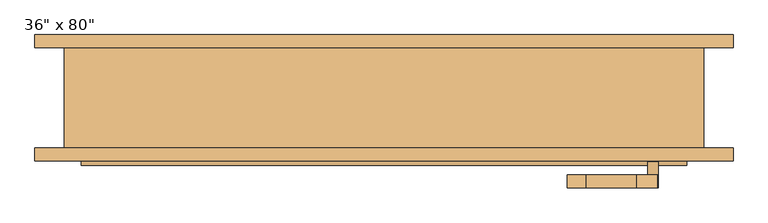
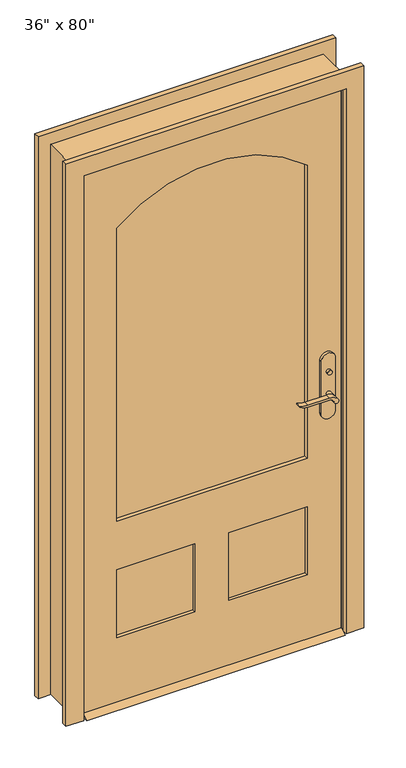
"""IFC4 building model written with IfcOpenShell, lengths in millimetres: door geometry."""

from ifc_helpers import new_model, si_unit, point, frame, frame_2d, origin, place, context, project, spatial, polyline, circle_curve, trimmed, segment, composite_curve, outline, extrude, faceted_brep, source, transform, mapped, element, save


def door_5d363d20(model_context):
    return source(origin(), model_context, "Body", "SolidModel", [
        extrude(outline(polyline([(-38.1, 12.7), (-12.7, 0.0), (-98.425, 0.0), (-73.025, 12.7), (-38.1, 12.7)])), frame((-457.2, 0.0, 0.0), z_axis=(1.0, 0.0, 0.0), x_axis=(0.0, 1.0, 0.0)), (0.0, 0.0, 1.0), 914.4),
        extrude(outline(polyline([(411.4, -18.1), (411.4, -28.1), (401.4, -28.1), (401.4, -18.1), (411.4, -18.1)])), frame((0.0, 0.0, 981.9), z_axis=(0.0, 0.0, 1.0), x_axis=(1.0, 0.0, 0.0)), (0.0, 0.0, 1.0), 30.0),
        extrude(outline(composite_curve([segment(trimmed(circle_curve(frame_2d((996.9, 406.4)), 8.0), [point((996.9, 398.4))], [point((996.9, 414.4))], False, "CARTESIAN"), True, "CONTINUOUS"), segment(trimmed(circle_curve(frame_2d((996.9, 406.4)), 8.0), [point((996.9, 414.4))], [point((996.9, 398.4))], False, "CARTESIAN"), True, "CONTINUOUS")], self_intersect=False)), frame((0.0, -93.025, 0.0), z_axis=(0.0, 1.0, 0.0), x_axis=(0.0, 0.0, 1.0)), (0.0, 0.0, 1.0), 10.0),
        extrude(outline(composite_curve([segment(trimmed(circle_curve(frame_2d((897.1555521, 382.7324871)), 37.2832219), [point((919.0523287, 412.9081363))], [point((934.4, 381.0325667))], False, "CARTESIAN"), True, "CONTINUOUS"), segment(polyline([(934.4, 381.0325667), (934.4, 304.7564091)]), True, "CONTINUOUS"), segment(trimmed(circle_curve(frame_2d((1017.6850638, 304.8227909)), 83.2850902), [point((934.4, 304.7564091))], [point((939.4, 276.4))], True, "CARTESIAN"), True, "CONTINUOUS"), segment(polyline([(939.4, 276.4), (936.6135558, 276.4)]), True, "CONTINUOUS"), segment(trimmed(circle_curve(frame_2d((986.6709207, 308.3396612)), 59.3791355), [point((936.6135558, 276.4))], [point((927.4, 304.7564091))], False, "CARTESIAN"), True, "CONTINUOUS"), segment(polyline([(927.4, 304.7564091), (927.4, 381.0138099)]), True, "CONTINUOUS"), segment(trimmed(circle_curve(frame_2d((909.2738613, 381.0138099)), 18.1261387), [point((927.4, 381.0138099))], [point((914.4, 398.4))], True, "CARTESIAN"), True, "CONTINUOUS"), segment(trimmed(circle_curve(frame_2d((914.4, 406.4)), 8.0), [point((914.4, 398.4))], [point((919.0523287, 412.9081363))], False, "CARTESIAN"), True, "CONTINUOUS")], self_intersect=False)), frame((0.0, 1.9, 0.0), z_axis=(0.0, 1.0, 0.0), x_axis=(0.0, 0.0, 1.0)), (0.0, 0.0, 1.0), 20.0),
        extrude(outline(composite_curve([segment(trimmed(circle_curve(frame_2d((914.4, 406.4)), 8.0), [point((914.3999903, 398.4))], [point((919.0523287, 412.9081363))], False, "CARTESIAN"), True, "CONTINUOUS"), segment(trimmed(circle_curve(frame_2d((897.1555521, 382.7324871)), 37.2832219), [point((919.0523287, 412.9081363))], [point((934.4, 381.0325667))], False, "CARTESIAN"), True, "CONTINUOUS"), segment(polyline([(934.4, 381.0325667), (934.4, 304.7564091)]), True, "CONTINUOUS"), segment(trimmed(circle_curve(frame_2d((1017.6850638, 304.8227909)), 83.2850902), [point((934.4, 304.7564091))], [point((939.4, 276.4))], True, "CARTESIAN"), True, "CONTINUOUS"), segment(polyline([(939.4, 276.4), (936.6135558, 276.4)]), True, "CONTINUOUS"), segment(trimmed(circle_curve(frame_2d((986.6709207, 308.3396612)), 59.3791355), [point((936.6135558, 276.4))], [point((927.4, 304.7564091))], False, "CARTESIAN"), True, "CONTINUOUS"), segment(polyline([(927.4, 304.7564091), (927.4, 381.0138122)]), True, "CONTINUOUS"), segment(trimmed(circle_curve(frame_2d((909.2738682, 381.0138122)), 18.1261318), [point((927.4, 381.0138122))], [point((914.3999903, 398.4))], True, "CARTESIAN"), True, "CONTINUOUS")], self_intersect=False)), frame((0.0, -133.025, 0.0), z_axis=(0.0, 1.0, 0.0), x_axis=(0.0, 0.0, 1.0)), (0.0, 0.0, 1.0), 20.0),
        extrude(outline(composite_curve([segment(trimmed(circle_curve(frame_2d((914.4, 406.4)), 8.0), [point((914.4, 398.4))], [point((914.4, 414.4))], False, "CARTESIAN"), True, "CONTINUOUS"), segment(trimmed(circle_curve(frame_2d((914.4, 406.4)), 8.0), [point((914.4, 414.4))], [point((914.4, 398.4))], False, "CARTESIAN"), True, "CONTINUOUS")], self_intersect=False)), frame((0.0, -28.1, 0.0), z_axis=(0.0, 1.0, 0.0), x_axis=(0.0, 0.0, 1.0)), (0.0, 0.0, 1.0), 30.0),
        extrude(outline(composite_curve([segment(trimmed(circle_curve(frame_2d((914.4, 406.4)), 8.0), [point((914.4, 398.4))], [point((914.4, 414.4))], False, "CARTESIAN"), True, "CONTINUOUS"), segment(trimmed(circle_curve(frame_2d((914.4, 406.4)), 8.0), [point((914.4, 414.4))], [point((914.4, 398.4))], False, "CARTESIAN"), True, "CONTINUOUS")], self_intersect=False)), frame((0.0, -113.025, 0.0), z_axis=(0.0, 1.0, 0.0), x_axis=(0.0, 0.0, 1.0)), (0.0, 0.0, 1.0), 30.0),
        extrude(outline(composite_curve([segment(polyline([(844.4, 431.4), (1039.4, 431.4)]), True, "CONTINUOUS"), segment(trimmed(circle_curve(frame_2d((1039.4, 406.4)), 25.0), [point((1039.4, 431.4))], [point((1039.4, 381.4))], False, "CARTESIAN"), True, "CONTINUOUS"), segment(polyline([(1039.4, 381.4), (844.4, 381.4)]), True, "CONTINUOUS"), segment(trimmed(circle_curve(frame_2d((844.4, 406.4)), 25.0), [point((844.4, 381.4))], [point((844.4, 431.4))], False, "CARTESIAN"), True, "CONTINUOUS")], self_intersect=False)), frame((0.0, -38.1, 0.0), z_axis=(0.0, 1.0, 0.0), x_axis=(0.0, 0.0, 1.0)), (0.0, 0.0, 1.0), 10.0),
        extrude(outline(composite_curve([segment(polyline([(844.4, 431.4), (1039.4, 431.4)]), True, "CONTINUOUS"), segment(trimmed(circle_curve(frame_2d((1039.4, 406.4)), 25.0), [point((1039.4, 431.4))], [point((1039.4, 381.4))], False, "CARTESIAN"), True, "CONTINUOUS"), segment(polyline([(1039.4, 381.4), (844.4, 381.4)]), True, "CONTINUOUS"), segment(trimmed(circle_curve(frame_2d((844.4, 406.4)), 25.0), [point((844.4, 381.4))], [point((844.4, 431.4))], False, "CARTESIAN"), True, "CONTINUOUS")], self_intersect=False)), frame((0.0, -83.025, 0.0), z_axis=(0.0, 1.0, 0.0), x_axis=(0.0, 0.0, 1.0)), (0.0, 0.0, 1.0), 10.0),
        extrude(outline(polyline([(2032.0, -457.2), (12.7, -457.2), (12.7, 457.2), (2032.0, 457.2), (2032.0, -457.2)]), holes=[composite_curve([segment(polyline([(688.975, -336.55), (1784.35, -336.55)]), True, "CONTINUOUS"), segment(trimmed(circle_curve(frame_2d((1401.92125, 0.0)), 509.42875), [point((1784.35, -336.55))], [point((1784.35, 336.55))], True, "CARTESIAN"), True, "CONTINUOUS"), segment(polyline([(1784.35, 336.55), (688.975, 336.55), (688.975, -336.55)]), True, "CONTINUOUS")], self_intersect=False), polyline([(508.0, -60.325), (254.0, -60.325), (254.0, -336.55), (508.0, -336.55), (508.0, -60.325)]), polyline([(508.0, 336.55), (254.0, 336.55), (254.0, 60.325), (508.0, 60.325), (508.0, 336.55)])]), frame((0.0, -73.025, 0.0), z_axis=(0.0, 1.0, 0.0), x_axis=(0.0, 0.0, 1.0)), (0.0, 0.0, 1.0), 34.925),
        faceted_brep([(482.6, -73.025, 0.0), (457.2, -73.025, 0.0), (457.2, -38.1, 0.0), (444.5, -38.1, 0.0), (444.5, -3.175, 0.0), (457.2, -3.175, 0.0), (457.2, 79.375, 0.0), (482.6, 79.375, 0.0), (482.6, 79.375, 2057.4), (482.6, -73.025, 2057.4), (457.2, 79.375, 2032.0), (-457.2, 79.375, 2032.0), (-457.2, 79.375, 0.0), (-482.6, 79.375, 0.0), (-482.6, 79.375, 2057.4), (457.2, -3.175, 2032.0), (444.5, -3.175, 2019.3), (-444.5, -3.175, 2019.3), (-444.5, -3.175, 0.0), (-457.2, -3.175, 0.0), (-457.2, -3.175, 2032.0), (444.5, -38.1, 2019.3), (457.2, -38.1, 2032.0), (-457.2, -38.1, 2032.0), (-457.2, -38.1, 0.0), (-444.5, -38.1, 0.0), (-444.5, -38.1, 2019.3), (457.2, -73.025, 2032.0), (-482.6, -73.025, 2057.4), (-482.6, -73.025, 0.0), (-457.2, -73.025, 0.0), (-457.2, -73.025, 2032.0)], [[[0, 1, 2, 3, 4, 5, 6, 7]], [[7, 8, 9, 0]], [[6, 10, 11, 12, 13, 14, 8, 7]], [[5, 15, 10, 6]], [[4, 16, 17, 18, 19, 20, 15, 5]], [[3, 21, 16, 4]], [[2, 22, 23, 24, 25, 26, 21, 3]], [[1, 27, 22, 2]], [[0, 9, 28, 29, 30, 31, 27, 1]], [[8, 14, 28, 9]], [[15, 20, 11, 10]], [[21, 26, 17, 16]], [[27, 31, 23, 22]], [[29, 13, 12, 19, 18, 25, 24, 30]], [[14, 13, 29, 28]], [[20, 19, 12, 11]], [[26, 25, 18, 17]], [[31, 30, 24, 23]]]),
        extrude(outline(polyline([(-60.325, -49.7416667), (-60.325, -61.3833333), (-336.55, -61.3833333), (-336.55, -49.7416667), (-60.325, -49.7416667)])), frame((0.0, 0.0, 254.0), z_axis=(0.0, 0.0, 1.0), x_axis=(1.0, 0.0, 0.0)), (0.0, 0.0, 1.0), 254.0),
        extrude(outline(polyline([(336.55, -49.7416667), (336.55, -61.3833333), (60.325, -61.3833333), (60.325, -49.7416667), (336.55, -49.7416667)])), frame((0.0, 0.0, 254.0), z_axis=(0.0, 0.0, 1.0), x_axis=(1.0, 0.0, 0.0)), (0.0, 0.0, 1.0), 254.0),
        extrude(outline(composite_curve([segment(polyline([(688.975, -336.55), (688.975, 336.55), (1784.35, 336.55)]), True, "CONTINUOUS"), segment(trimmed(circle_curve(frame_2d((1401.92125, 0.0)), 509.42875), [point((1784.35, 336.55))], [point((1784.35, -336.55))], False, "CARTESIAN"), True, "CONTINUOUS"), segment(polyline([(1784.35, -336.55), (688.975, -336.55)]), True, "CONTINUOUS")], self_intersect=False)), frame((0.0, -59.055, 0.0), z_axis=(0.0, 1.0, 0.0), x_axis=(0.0, 0.0, 1.0)), (0.0, 0.0, 1.0), 6.985),
        extrude(outline(polyline([(0.0, -463.55), (2038.35, -463.55), (2038.35, 463.55), (0.0, 463.55), (0.0, 527.05), (2101.85, 527.05), (2101.85, -527.05), (0.0, -527.05), (0.0, -463.55)])), frame((0.0, 79.375, 0.0), z_axis=(0.0, 1.0, 0.0), x_axis=(0.0, 0.0, 1.0)), (0.0, 0.0, 1.0), 19.05),
        extrude(outline(polyline([(0.0, -463.55), (2038.35, -463.55), (2038.35, 463.55), (0.0, 463.55), (0.0, 527.05), (2101.85, 527.05), (2101.85, -527.05), (0.0, -527.05), (0.0, -463.55)])), frame((0.0, -92.075, 0.0), z_axis=(0.0, 1.0, 0.0), x_axis=(0.0, 0.0, 1.0)), (0.0, 0.0, 1.0), 19.05),
    ])


if __name__ == "__main__":
    model = new_model("IFC4")
    model_context = context("Model", 3, world=origin())
    ifc_project = project(units=[si_unit("LENGTHUNIT", "METRE", prefix="MILLI")], contexts=[model_context])
    site = spatial("IfcSite", under=ifc_project)
    building = spatial("IfcBuilding", under=site)
    placement = place(None, origin())
    door_shape = door_5d363d20(model_context)
    element("IfcDoor", 1, ObjectType="36\" x 80\"", at=placement, inside=building, context=model_context, shape_type="MappedRepresentation", body=[
        mapped(door_shape, transform((0.0, 0.0, 0.0), x_axis=(1.0, 0.0, 0.0), y_axis=(0.0, 1.0, 0.0), z_axis=(0.0, 0.0, 1.0))),
    ])
    save(model, "model.ifc")

# Revit data of these elements
# Type "36\" x 80\""
#   Type Mark = "15"
#   Assembly Code = "B2030100"
#   Analytic Construction = "French door, wood frame with single glass"
#   Threshold Offset [instance default] = 0' - 0 1/2"
#   Thickness = 0' - 1 3/8"
#   Thermal Resistance (R) = 1.0696 (h·ft²·°F)/BTU
#   Swing Angle [instance default] = 90.00°
#   Stiles = 0' - 4 3/4"
#   Rough Width = 3' - 2"
#   Rough Height = 6' - 9"
#   Radius = 1' - 8.05625"
#   Lock Rail = 0' - 7 1/8"
#   Height = 6' - 8"
#   Width = 3' - 0"
#   Heat Transfer Coefficient (U) = 0.9350 BTU/(h·ft²·°F)
#   Door Offset [instance default] = 0' - 0"
#   Bottom Rail = 0' - 9 1/2"
#   Threshold [instance default] = yes
#   Function = 1
#   Exterior Trim [instance default] = yes
#   Trim Material = Cherry
#   Threshold Material = Cherry
#   Panel Material = Cherry
#   Glazing = Glass
#   Frame Material = Cherry
#   Door Handle Material = Aluminum
#   Visual Light Transmittance = 0
#   Solar Heat Gain Coefficient = 0
#   Wall Closure = (empty or 0)
#   Construction Type = (empty or 0)
# Element 1 (IfcDoor, "36\" x 80\"")
#   Materials on its faces: "Cherry", "Aluminum", "Glass"
# Materials
#   "Cherry": class "Wood", colour RGB 226 177 128, transparency 0, Description = "Prunus Serotina", Cost = 0
#   "Glass": class "Glass", colour RGB 0 128 192, transparency 0.75, Description = "Soda Lime Glass", Cost = 0
#   "Aluminum": class "Metal", colour RGB 247 247 247, transparency 0, Description = "Aluminum 6061", Cost = 0
